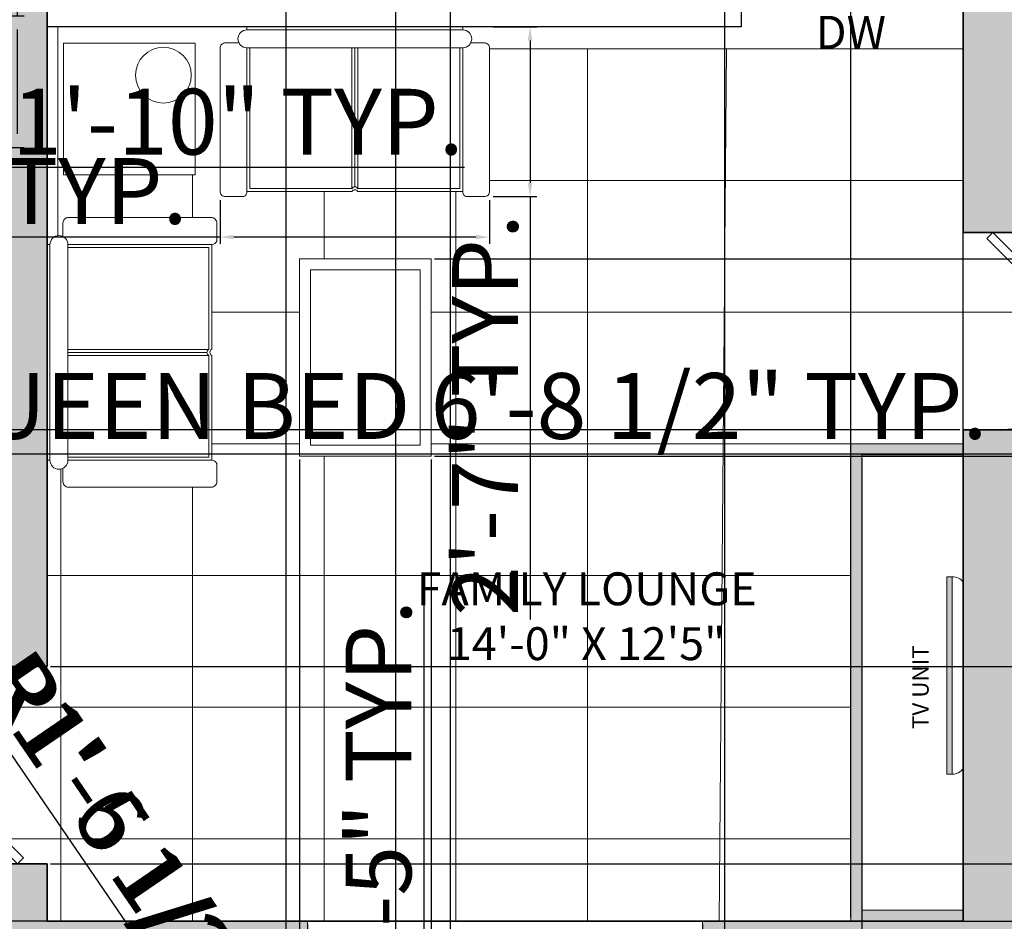
# Model space of a CAD drawing. Units: millimetres. Extents: x 542930 to 543750, y 628093 to 628738.
# Tile 6 of 14: x 543153 to 543333, y 628350 to 628514. Entities that reach past the tile are written whole.
import ezdxf

# ---------------------------------------------------------------- set-up
doc = ezdxf.new("R2010")
doc.units = ezdxf.units.MM
for name, color, linetype, lineweight in [('A-ANNO-DIMS', 2, 'Continuous', 18), ('A-EQPM', 9, 'Continuous', 18), ('A-EQPM-PATT', 9, 'Continuous', 13), ('A-FLOR-STRS', 7, 'Continuous', 25), ('A-FURN', 8, 'Continuous', 18), ('A-FURN-MILL', 8, 'Continuous', 18), ('A-FURN-PATT', 9, 'Continuous', 13), ('A-WALL', 7, 'Continuous', 35), ('DOORS', 30, 'Continuous', 18)]:
    doc.layers.add(name, color=color, linetype=linetype, lineweight=lineweight)
for name, color, linetype, lineweight, true_color in [('A-ANNO-TEXT', 40, 'Continuous', 18, 0xf8d731), ('A-AREA-IDEN', 40, 'Continuous', 18, 0xf8d731), ('A-FLOR-PATT', 241, 'Continuous', 13, 0xf7abae), ('A-WALL-PATT', 251, 'Continuous', 13, 0x636466)]:
    doc.layers.add(name, color=color, linetype=linetype, lineweight=lineweight, true_color=true_color)
doc.styles.get("Standard").update_dxf_attribs({"font": 'arial.ttf'})
doc.dimstyles.new('ISO-25', dxfattribs={"dimtxt": 12, "dimasz": 2.5, "dimexe": 1.25, "dimexo": 0.625, "dimtad": 1, "dimdec": 0, "dimlunit": 3, "dimtxsty": 'Standard', "dimcen": 2.5, "dimadec": 0, "dimazin": 0, "dimtfac": 1, "dimtdec": 0, "dimtmove": 0, "dimatfit": 3, "dimfxl": 1, "dimarcsym": 0})

# ---------------------------------------------------------------- blocks, each defined once
blk = doc.blocks.new('*U2')
for p, q in [((0, 0), (0, -6)), ((40, 0), (40, -6))]:
    blk.add_line(p, q)
blk.add_lwpolyline([(0, 0), (28.28, 28.28), (29.52, 27.05), (1.24, -1.24)], close=True)
blk.add_arc((0, 0), 40, 0, 45)
blk = doc.blocks.new('*U4')
for p, q in [((0, 0), (0, -6)), ((40, 0), (40, -6))]:
    blk.add_line(p, q)
blk.add_lwpolyline([(0, 0), (28.28, 28.28), (29.52, 27.05), (1.24, -1.24)], close=True)
blk.add_arc((0, 0), 40, 0, 45)
blk = doc.blocks.new('sofa')
for p, q in [((543001.62, 628230.38), (543001.62, 628182.38)), ((543010.62, 628230.38), (543045.62, 628230.38)), ((543091.62, 628230.38), (543091.62, 628182.38)), ((543045.62, 628229.38), (543045.62, 628182.38)), ((543046.62, 628228.78), (543046.62, 628182.38)), ((543010.62, 628176.38), (543082.62, 628176.38))]:
    blk.add_line(p, q)
for points in [[(543009.53, 628232.06), (543003.46, 628232.06, 0.414214), (543001.62, 628230.23)], [(543045.62, 628230.38, 0.623864), (543047.62, 628230.38), (543082.62, 628230.38), (543082.62, 628182.38), (543010.62, 628182.38), (543010.62, 628230.38, 0.297291), (543009.53, 628232.06)], [(543083.72, 628232.06, 0.297291), (543082.62, 628230.38), (543082.62, 628182.38)], [(543091.62, 628230.23, 0.414214), (543089.79, 628232.06), (543083.72, 628232.06)], [(543001.62, 628182.54, 0.414214), (543003.46, 628180.7), (543007.93, 628180.7)], [(543082.62, 628182.38, -1), (543082.62, 628176.38), (543082.62, 628175.38), (543010.62, 628175.38), (543010.62, 628176.38, -1), (543010.62, 628182.38)], [(543085.32, 628180.7), (543089.79, 628180.7, 0.414214), (543091.62, 628182.54)]]:
    blk.add_lwpolyline(points, format="xyb")
for points in [[(543011.62, 628182.38), (543011.62, 628229.38), (543045.62, 628229.38), (543045.62, 628229.4)], [(543047.62, 628182.38), (543047.62, 628229.38), (543047.62, 628229.4)], [(543047.62, 628229.38), (543081.62, 628229.38), (543081.62, 628182.38)]]:
    blk.add_lwpolyline(points)
blk.add_arc((543046.62, 628229.89), 1.11, 206.0829, 333.9171)
blk = doc.blocks.new('*D33')
at = {"layer": 'A-ANNO-DIMS', "color": 0, "lineweight": -2, "transparency": 16777216}
for p, q in [((543189.7, 628481.25), (543189.7, 628473.25)), ((543238.84, 628481.25), (543238.84, 628473.25)), ((543189.7, 628474.5), (543062.56, 628474.5)), ((543236.34, 628474.5), (543192.2, 628474.5))]:
    blk.add_line(p, q, dxfattribs=at)
at = {"layer": 'A-ANNO-DIMS', "color": 0, "transparency": 16777216}
for points in [[(543192.2, 628474.92), (543192.2, 628474.09), (543189.7, 628474.5)], [(543236.34, 628474.92), (543236.34, 628474.09), (543238.84, 628474.5)]]:
    blk.add_solid(points, dxfattribs=at)
at = {"layer": 'Defpoints', "color": 0, "transparency": 16777216}
for p in [(543189.7, 628481.87), (543238.84, 628481.87), (543189.7, 628474.5)]:
    blk.add_point(p, dxfattribs=at)
at = {"layer": 'A-ANNO-DIMS', "color": 0, "transparency": 16777216, "insert": (543124.88, 628481.34), "char_height": 12, "attachment_point": 5}
blk.add_mtext('SOFA 4\'-1" TYP.', dxfattribs=at)
blk = doc.blocks.new('*D34')
at = {"layer": 'A-ANNO-DIMS', "color": 0, "lineweight": -2, "transparency": 16777216}
for p, q in [((543239.47, 628512.83), (543247.47, 628512.83)), ((543246.22, 628510.33), (543246.22, 628484.37)), ((543239.47, 628481.87), (543247.47, 628481.87)), ((543246.22, 628481.87), (543246.22, 628404.77))]:
    blk.add_line(p, q, dxfattribs=at)
at = {"layer": 'A-ANNO-DIMS', "color": 0, "transparency": 16777216}
for points in [[(543245.8, 628510.33), (543246.63, 628510.33), (543246.22, 628512.83)], [(543245.8, 628484.37), (543246.63, 628484.37), (543246.22, 628481.87)]]:
    blk.add_solid(points, dxfattribs=at)
at = {"layer": 'Defpoints', "color": 0, "transparency": 16777216}
for p in [(543238.84, 628512.83), (543238.84, 628481.87), (543246.22, 628481.87)]:
    blk.add_point(p, dxfattribs=at)
at = {"layer": 'A-ANNO-DIMS', "color": 0, "transparency": 16777216, "insert": (543239.56, 628442.07), "char_height": 12, "attachment_point": 5, "rotation": 90}
blk.add_mtext('2\'-7" TYP.', dxfattribs=at)
blk = doc.blocks.new('*D37')
at = {"layer": 'A-ANNO-DIMS', "color": 0, "lineweight": -2, "transparency": 16777216}
for p, q in [((543337.17, 628423.55), (543337.17, 628436.21)), ((543417.44, 628423.55), (543417.44, 628436.21)), ((543337.17, 628434.96), (543128.93, 628434.96)), ((543414.94, 628434.96), (543339.67, 628434.96))]:
    blk.add_line(p, q, dxfattribs=at)
at = {"layer": 'A-ANNO-DIMS', "color": 0, "transparency": 16777216}
for points in [[(543339.67, 628435.38), (543339.67, 628434.55), (543337.17, 628434.96)], [(543414.94, 628435.38), (543414.94, 628434.55), (543417.44, 628434.96)]]:
    blk.add_solid(points, dxfattribs=at)
at = {"layer": 'Defpoints', "color": 0, "transparency": 16777216}
for p in [(543337.17, 628434.96), (543337.17, 628422.92), (543417.44, 628422.92)]:
    blk.add_point(p, dxfattribs=at)
at = {"layer": 'A-ANNO-DIMS', "color": 0, "transparency": 16777216, "insert": (543231.8, 628442.16), "char_height": 12, "attachment_point": 5}
blk.add_mtext('QUEEN BED 6\'-8 1/2" TYP.', dxfattribs=at)
blk = doc.blocks.new('*D42')
at = {"layer": 'A-ANNO-DIMS', "color": 0, "lineweight": -2, "transparency": 16777216}
for p, q in [((543226.89, 628332.06), (543226.89, 628408.95)), ((543221.13, 628332.06), (543228.14, 628332.06)), ((543226.89, 628293.55), (543226.89, 628329.56)), ((543221.13, 628291.05), (543228.14, 628291.05))]:
    blk.add_line(p, q, dxfattribs=at)
at = {"layer": 'A-ANNO-DIMS', "color": 0, "transparency": 16777216}
for points in [[(543226.47, 628329.56), (543227.3, 628329.56), (543226.89, 628332.06)], [(543226.47, 628293.55), (543227.3, 628293.55), (543226.89, 628291.05)]]:
    blk.add_solid(points, dxfattribs=at)
at = {"layer": 'Defpoints', "color": 0, "transparency": 16777216}
for p in [(543220.5, 628332.06), (543226.89, 628332.06), (543220.5, 628291.05)]:
    blk.add_point(p, dxfattribs=at)
at = {"layer": 'A-ANNO-DIMS', "color": 0, "transparency": 16777216, "insert": (543220.13, 628371.75), "char_height": 12, "attachment_point": 5, "rotation": 90}
blk.add_mtext('3\'-5" TYP.', dxfattribs=at)
blk = doc.blocks.new('*D55')
at = {"layer": 'A-ANNO-DIMS', "color": 0, "lineweight": -2, "transparency": 16777216}
for p, q in [((543152.77, 628514.83), (543152.77, 628679.13)), ((543149.79, 628514.83), (543154.02, 628514.83)), ((543152.77, 628493.33), (543152.77, 628512.33)), ((543149.79, 628490.83), (543154.02, 628490.83))]:
    blk.add_line(p, q, dxfattribs=at)
at = {"layer": 'A-ANNO-DIMS', "color": 0, "transparency": 16777216}
for points in [[(543152.35, 628512.33), (543153.18, 628512.33), (543152.77, 628514.83)], [(543152.35, 628493.33), (543153.18, 628493.33), (543152.77, 628490.83)]]:
    blk.add_solid(points, dxfattribs=at)
at = {"layer": 'Defpoints', "color": 0, "transparency": 16777216}
for p in [(543149.17, 628514.83), (543152.77, 628514.83), (543149.17, 628490.83)]:
    blk.add_point(p, dxfattribs=at)
at = {"layer": 'A-ANNO-DIMS', "color": 0, "transparency": 16777216, "insert": (543145.93, 628598.23), "char_height": 12, "attachment_point": 5, "rotation": 90}
blk.add_mtext('COUNTER 2\'-0" TYP.', dxfattribs=at)
blk = doc.blocks.new('*D56')
at = {"layer": 'A-ANNO-DIMS', "color": 0, "lineweight": -2, "transparency": 16777216}
for p, q in [((543127.17, 628490.2), (543127.17, 628485.98)), ((543149.17, 628490.2), (543149.17, 628485.98)), ((543129.67, 628487.23), (543146.67, 628487.23)), ((543149.17, 628487.23), (543234.26, 628487.23))]:
    blk.add_line(p, q, dxfattribs=at)
at = {"layer": 'A-ANNO-DIMS', "color": 0, "transparency": 16777216}
for points in [[(543129.67, 628487.64), (543129.67, 628486.81), (543127.17, 628487.23)], [(543146.67, 628487.64), (543146.67, 628486.81), (543149.17, 628487.23)]]:
    blk.add_solid(points, dxfattribs=at)
at = {"layer": 'Defpoints', "color": 0, "transparency": 16777216}
for p in [(543127.17, 628490.83), (543149.17, 628490.83), (543149.17, 628487.23)]:
    blk.add_point(p, dxfattribs=at)
at = {"layer": 'A-ANNO-DIMS', "color": 0, "transparency": 16777216, "insert": (543192.96, 628493.98), "char_height": 12, "attachment_point": 5}
blk.add_mtext('1\'-10" TYP.', dxfattribs=at)
blk = doc.blocks.new('*D71')
at = {"layer": 'A-ANNO-DIMS', "color": 0, "lineweight": -2, "transparency": 16777216}
for p, q in [((543201.67, 628544.2), (543201.67, 628103.84)), ((543281.67, 628544.2), (543281.67, 628103.84)), ((543204.17, 628105.09), (543279.17, 628105.09))]:
    blk.add_line(p, q, dxfattribs=at)
at = {"layer": 'A-ANNO-DIMS', "color": 0, "transparency": 16777216}
for points in [[(543204.17, 628105.5), (543204.17, 628104.67), (543201.67, 628105.09)], [(543279.17, 628105.5), (543279.17, 628104.67), (543281.67, 628105.09)]]:
    blk.add_solid(points, dxfattribs=at)
at = {"layer": 'Defpoints', "color": 0, "transparency": 16777216}
for p in [(543201.67, 628544.83), (543281.67, 628544.83), (543281.67, 628105.09)]:
    blk.add_point(p, dxfattribs=at)
at = {"layer": 'A-ANNO-DIMS', "color": 0, "transparency": 16777216, "insert": (543241.67, 628111.84), "char_height": 12, "attachment_point": 5}
blk.add_mtext('6\'-8"', dxfattribs=at)
blk = doc.blocks.new('*D73')
at = {"layer": 'A-ANNO-DIMS', "color": 0, "lineweight": -2, "transparency": 16777216}
for p, q in [((543158.79, 628396.23), (543537.81, 628396.23)), ((543536.56, 628362.73), (543536.56, 628393.73)), ((543158.79, 628360.23), (543537.81, 628360.23))]:
    blk.add_line(p, q, dxfattribs=at)
at = {"layer": 'A-ANNO-DIMS', "color": 0, "transparency": 16777216}
for points in [[(543536.15, 628393.73), (543536.98, 628393.73), (543536.56, 628396.23)], [(543536.15, 628362.73), (543536.98, 628362.73), (543536.56, 628360.23)]]:
    blk.add_solid(points, dxfattribs=at)
at = {"layer": 'Defpoints', "color": 0, "transparency": 16777216}
for p in [(543158.17, 628396.23), (543536.56, 628396.23), (543158.17, 628360.23)]:
    blk.add_point(p, dxfattribs=at)
at = {"layer": 'A-ANNO-DIMS', "color": 0, "transparency": 16777216, "insert": (543529.81, 628378.23), "char_height": 12, "attachment_point": 5, "rotation": 90}
blk.add_mtext('3\'-0"', dxfattribs=at)
blk = doc.blocks.new('*D74')
at = {"layer": 'A-ANNO-DIMS', "color": 0, "lineweight": -2, "transparency": 16777216}
for p, q in [((543536.56, 628360.23), (543536.56, 628433.16)), ((543158.79, 628360.23), (543537.81, 628360.23)), ((543536.56, 628352.33), (543536.56, 628357.73)), ((543158.79, 628349.83), (543537.81, 628349.83))]:
    blk.add_line(p, q, dxfattribs=at)
at = {"layer": 'A-ANNO-DIMS', "color": 0, "transparency": 16777216}
for points in [[(543536.15, 628357.73), (543536.98, 628357.73), (543536.56, 628360.23)], [(543536.15, 628352.33), (543536.98, 628352.33), (543536.56, 628349.83)]]:
    blk.add_solid(points, dxfattribs=at)
at = {"layer": 'Defpoints', "color": 0, "transparency": 16777216}
for p in [(543158.17, 628360.23), (543536.56, 628360.23), (543158.17, 628349.83)]:
    blk.add_point(p, dxfattribs=at)
at = {"layer": 'A-ANNO-DIMS', "color": 0, "transparency": 16777216, "insert": (543529.73, 628397.95), "char_height": 12, "attachment_point": 5, "rotation": 90}
blk.add_mtext('0\'-10 1/2"', dxfattribs=at)
blk = doc.blocks.new('*D75')
at = {"layer": 'A-ANNO-DIMS', "color": 0, "lineweight": -2, "transparency": 16777216}
for p, q in [((543324.54, 628439.36), (542953.72, 628439.36)), ((542954.97, 628352.33), (542954.97, 628436.86)), ((543324.54, 628349.83), (542953.72, 628349.83))]:
    blk.add_line(p, q, dxfattribs=at)
at = {"layer": 'A-ANNO-DIMS', "color": 0, "transparency": 16777216}
for points in [[(542954.55, 628436.86), (542955.38, 628436.86), (542954.97, 628439.36)], [(542954.55, 628352.33), (542955.38, 628352.33), (542954.97, 628349.83)]]:
    blk.add_solid(points, dxfattribs=at)
at = {"layer": 'Defpoints', "color": 0, "transparency": 16777216}
for p in [(542954.97, 628439.36), (543325.17, 628439.36), (543325.17, 628349.83)]:
    blk.add_point(p, dxfattribs=at)
at = {"layer": 'A-ANNO-DIMS', "color": 0, "transparency": 16777216, "insert": (542948.14, 628394.6), "char_height": 12, "attachment_point": 5, "rotation": 90}
blk.add_mtext('7\'-5 1/2"', dxfattribs=at)
blk = doc.blocks.new('*D76')
at = {"layer": 'A-ANNO-DIMS', "color": 0, "lineweight": -2, "transparency": 16777216}
for p, q in [((543205.67, 628349.2), (543205.67, 628103.84)), ((543277.67, 628349.2), (543277.67, 628103.84)), ((543208.17, 628105.09), (543275.17, 628105.09))]:
    blk.add_line(p, q, dxfattribs=at)
at = {"layer": 'A-ANNO-DIMS', "color": 0, "transparency": 16777216}
for points in [[(543208.17, 628105.5), (543208.17, 628104.67), (543205.67, 628105.09)], [(543275.17, 628105.5), (543275.17, 628104.67), (543277.67, 628105.09)]]:
    blk.add_solid(points, dxfattribs=at)
at = {"layer": 'Defpoints', "color": 0, "transparency": 16777216}
for p in [(543205.67, 628349.83), (543277.67, 628349.83), (543277.67, 628105.09)]:
    blk.add_point(p, dxfattribs=at)
at = {"layer": 'A-ANNO-DIMS', "color": 0, "transparency": 16777216, "insert": (543241.67, 628111.84), "char_height": 12, "attachment_point": 5}
blk.add_mtext('6\'-0"', dxfattribs=at)
blk = doc.blocks.new('*D78')
at = {"layer": 'A-ANNO-DIMS', "color": 0, "lineweight": -2, "transparency": 16777216}
for p, q in [((543304.67, 628350.45), (543304.67, 628619.78)), ((543307.17, 628618.53), (543322.67, 628618.53)), ((543325.17, 628350.45), (543325.17, 628619.78)), ((543325.17, 628618.53), (543387.65, 628618.53))]:
    blk.add_line(p, q, dxfattribs=at)
at = {"layer": 'A-ANNO-DIMS', "color": 0, "transparency": 16777216}
for points in [[(543307.17, 628618.94), (543307.17, 628618.11), (543304.67, 628618.53)], [(543322.67, 628618.94), (543322.67, 628618.11), (543325.17, 628618.53)]]:
    blk.add_solid(points, dxfattribs=at)
at = {"layer": 'Defpoints', "color": 0, "transparency": 16777216}
for p in [(543325.17, 628618.53), (543304.67, 628349.83), (543325.17, 628349.83)]:
    blk.add_point(p, dxfattribs=at)
at = {"layer": 'A-ANNO-DIMS', "color": 0, "transparency": 16777216, "insert": (543357.66, 628625.36), "char_height": 12, "attachment_point": 5}
blk.add_mtext('1\'-8 1/2"', dxfattribs=at)
blk = doc.blocks.new('*D79')
at = {"layer": 'A-ANNO-DIMS', "color": 0, "lineweight": -2, "transparency": 16777216}
for p, q in [((543204.19, 628433.96), (543204.19, 628103.84)), ((543228.16, 628433.96), (543228.16, 628103.84)), ((543206.69, 628105.09), (543225.66, 628105.09)), ((543228.16, 628105.09), (543264.02, 628105.09))]:
    blk.add_line(p, q, dxfattribs=at)
at = {"layer": 'A-ANNO-DIMS', "color": 0, "transparency": 16777216}
for points in [[(543206.69, 628105.5), (543206.69, 628104.67), (543204.19, 628105.09)], [(543225.66, 628105.5), (543225.66, 628104.67), (543228.16, 628105.09)]]:
    blk.add_solid(points, dxfattribs=at)
at = {"layer": 'Defpoints', "color": 0, "transparency": 16777216}
for p in [(543204.19, 628434.59), (543228.16, 628434.59), (543228.16, 628105.09)]:
    blk.add_point(p, dxfattribs=at)
at = {"layer": 'A-ANNO-DIMS', "color": 0, "transparency": 16777216, "insert": (543247.34, 628111.84), "char_height": 12, "attachment_point": 5}
blk.add_mtext('2\'-0"', dxfattribs=at)
blk = doc.blocks.new('*D80')
at = {"layer": 'A-ANNO-DIMS', "color": 0, "lineweight": -2, "transparency": 16777216}
for p, q in [((543228.79, 628470.52), (543537.81, 628470.52)), ((543536.56, 628437.09), (543536.56, 628468.02)), ((543228.79, 628434.59), (543537.81, 628434.59))]:
    blk.add_line(p, q, dxfattribs=at)
at = {"layer": 'A-ANNO-DIMS', "color": 0, "transparency": 16777216}
for points in [[(543536.15, 628468.02), (543536.98, 628468.02), (543536.56, 628470.52)], [(543536.15, 628437.09), (543536.98, 628437.09), (543536.56, 628434.59)]]:
    blk.add_solid(points, dxfattribs=at)
at = {"layer": 'Defpoints', "color": 0, "transparency": 16777216}
for p in [(543228.16, 628470.52), (543536.56, 628470.52), (543228.16, 628434.59)]:
    blk.add_point(p, dxfattribs=at)
at = {"layer": 'A-ANNO-DIMS', "color": 0, "transparency": 16777216, "insert": (543529.81, 628452.55), "char_height": 12, "attachment_point": 5, "rotation": 90}
blk.add_mtext('3\'-0"', dxfattribs=at)
blk = doc.blocks.new('*D81')
at = {"layer": 'A-ANNO-DIMS', "color": 0, "lineweight": -2, "transparency": 16777216}
for p, q in [((543228.16, 628433.96), (543228.16, 628103.84)), ((543306.67, 628434.2), (543306.67, 628103.84)), ((543230.66, 628105.09), (543304.17, 628105.09))]:
    blk.add_line(p, q, dxfattribs=at)
at = {"layer": 'A-ANNO-DIMS', "color": 0, "transparency": 16777216}
for points in [[(543230.66, 628105.5), (543230.66, 628104.67), (543228.16, 628105.09)], [(543304.17, 628105.5), (543304.17, 628104.67), (543306.67, 628105.09)]]:
    blk.add_solid(points, dxfattribs=at)
at = {"layer": 'Defpoints', "color": 0, "transparency": 16777216}
for p in [(543228.16, 628434.59), (543306.67, 628434.83), (543306.67, 628105.09)]:
    blk.add_point(p, dxfattribs=at)
at = {"layer": 'A-ANNO-DIMS', "color": 0, "transparency": 16777216, "insert": (543267.41, 628111.92), "char_height": 12, "attachment_point": 5}
blk.add_mtext('6\'-6 1/2"', dxfattribs=at)
blk = doc.blocks.new('*D87')
at = {"layer": 'A-ANNO-DIMS', "color": 0, "lineweight": -2, "transparency": 16777216}
for p, q in [((543221.67, 628580.2), (543221.67, 628103.84)), ((543231.67, 628580.2), (543231.67, 628103.84)), ((543224.17, 628105.09), (543229.17, 628105.09)), ((543231.67, 628105.09), (543276.64, 628105.09))]:
    blk.add_line(p, q, dxfattribs=at)
at = {"layer": 'A-ANNO-DIMS', "color": 0, "transparency": 16777216}
for points in [[(543224.17, 628105.5), (543224.17, 628104.67), (543221.67, 628105.09)], [(543229.17, 628105.5), (543229.17, 628104.67), (543231.67, 628105.09)]]:
    blk.add_solid(points, dxfattribs=at)
at = {"layer": 'Defpoints', "color": 0, "transparency": 16777216}
for p in [(543221.67, 628580.83), (543231.67, 628580.83), (543231.67, 628105.09)]:
    blk.add_point(p, dxfattribs=at)
at = {"layer": 'A-ANNO-DIMS', "color": 0, "transparency": 16777216, "insert": (543255.4, 628111.84), "char_height": 12, "attachment_point": 5}
blk.add_mtext('0\'-10"', dxfattribs=at)
blk = doc.blocks.new('*D92')
at = {"layer": 'A-ANNO-DIMS', "color": 0, "lineweight": -2, "transparency": 16777216}
for p, q in [((543166.68, 628358.16), (543206.81, 628299.51)), ((543246.12, 628242.05), (543208.22, 628297.45))]:
    blk.add_line(p, q, dxfattribs=at)
at = {"layer": 'A-ANNO-DIMS', "color": 0, "transparency": 16777216}
blk.add_solid([(543208.57, 628297.68), (543207.88, 628297.21), (543206.81, 628299.51)], dxfattribs=at)
at = {"layer": 'Defpoints', "color": 0, "transparency": 16777216}
for p in [(543166.68, 628358.16), (543206.81, 628299.51)]:
    blk.add_point(p, dxfattribs=at)
at = {"layer": 'A-ANNO-DIMS', "color": 0, "transparency": 16777216, "insert": (543236.46, 628268.13), "char_height": 12, "attachment_point": 5, "rotation": 304.379}
blk.add_mtext('R5\'-11"', dxfattribs=at)
blk = doc.blocks.new('*D94')
at = {"layer": 'A-ANNO-DIMS', "color": 0, "lineweight": -2, "transparency": 16777216}
for p, q in [((543143.96, 628391.37), (543186.37, 628329.39)), ((543198.34, 628311.9), (543187.78, 628327.33))]:
    blk.add_line(p, q, dxfattribs=at)
at = {"layer": 'A-ANNO-DIMS', "color": 0, "transparency": 16777216}
blk.add_solid([(543186.71, 628329.63), (543186.02, 628329.15), (543187.78, 628327.33)], dxfattribs=at)
at = {"layer": 'Defpoints', "color": 0, "transparency": 16777216}
for p in [(543187.78, 628327.33), (543198.34, 628311.9)]:
    blk.add_point(p, dxfattribs=at)
at = {"layer": 'A-ANNO-DIMS', "color": 0, "transparency": 16777216, "insert": (543170.1, 628365.27), "char_height": 12, "attachment_point": 5, "rotation": 304.3793}
blk.add_mtext('R1\'-6 1/2"', dxfattribs=at)
blk = doc.blocks.new('*D95')
at = {"layer": 'A-ANNO-DIMS', "color": 0, "lineweight": -2, "transparency": 16777216}
for p, q in [((543144.53, 628390.54), (543186.93, 628328.57)), ((543198.34, 628311.9), (543188.34, 628326.5))]:
    blk.add_line(p, q, dxfattribs=at)
at = {"layer": 'A-ANNO-DIMS', "color": 0, "transparency": 16777216}
blk.add_solid([(543187.28, 628328.8), (543186.59, 628328.33), (543188.34, 628326.5)], dxfattribs=at)
at = {"layer": 'Defpoints', "color": 0, "transparency": 16777216}
for p in [(543188.34, 628326.5), (543198.34, 628311.9)]:
    blk.add_point(p, dxfattribs=at)
at = {"layer": 'A-ANNO-DIMS', "color": 0, "transparency": 16777216, "insert": (543170.66, 628364.44), "char_height": 12, "attachment_point": 5, "rotation": 304.3778}
blk.add_mtext('R1\'-5 1/2"', dxfattribs=at)

msp = doc.modelspace()

# ---------------------------------------------------------------- hatches: boundary and pattern name
at = {"layer": 'A-EQPM-PATT'}
h = msp.add_hatch(color=256, dxfattribs=at)
h.dxf.hatch_style = 1
h.paths.add_polyline_path([(543323.17, 628412.6), (543322.17, 628412.6), (543322.17, 628376.6), (543323.17, 628376.6)])
at = {"layer": 'A-FURN-PATT'}
h = msp.add_hatch(color=256, dxfattribs=at)
h.dxf.hatch_style = 1
h.paths.add_polyline_path([(543306.67, 628434.83), (543325.17, 628434.83), (543325.17, 628436.83), (543304.67, 628436.83), (543304.67, 628349.83), (543325.17, 628349.83), (543325.17, 628351.83), (543306.67, 628351.83)])
at = {"layer": 'A-WALL-PATT'}
h = msp.add_hatch(color=256, dxfattribs=at)
h.dxf.hatch_style = 1
h.paths.add_polyline_path([(543158.17, 628580.83), (543211.67, 628580.83), (543211.67, 628589.83), (543137.07, 628589.83), (543137.07, 628580.83), (543149.17, 628580.83), (543149.17, 628490.83), (543073.17, 628490.83), (543073.17, 628496.14), (543068.67, 628496.14), (543068.67, 628490.83), (543064.67, 628490.83), (543064.67, 628481.83), (543149.17, 628481.83), (543149.17, 628396.23), (543158.17, 628396.23)])
h = msp.add_hatch(color=256, dxfattribs=at)
h.dxf.hatch_style = 1
h.paths.add_polyline_path([(543454.53, 628589.83), (543271.67, 628589.83), (543271.67, 628580.83), (543325.17, 628580.83), (543325.17, 628475.36), (543334.17, 628475.36), (543334.17, 628481.83), (543370.17, 628481.83), (543370.17, 628490.83), (543334.17, 628490.83), (543334.17, 628580.83), (543410.17, 628580.83), (543410.17, 628524.86), (543414.67, 628524.86), (543414.67, 628580.83), (543454.53, 628580.83)])
h = msp.add_hatch(color=256, dxfattribs=at)
h.dxf.hatch_style = 1
h.paths.add_polyline_path([(543388.65, 628262.83), (543374.28, 628262.83), (543334.17, 628262.83), (543334.17, 628439.36), (543325.17, 628439.36), (543325.17, 628349.83), (543277.67, 628349.83), (543277.67, 628340.83), (543325.17, 628340.83), (543325.17, 628253.83), (543388.65, 628253.83)])
h = msp.add_hatch(color=256, dxfattribs=at)
h.dxf.hatch_style = 1
h.paths.add_polyline_path([(543158.17, 628340.83), (543205.67, 628340.83), (543205.67, 628349.83), (543158.17, 628349.83), (543158.17, 628360.23), (543149.17, 628360.23), (543149.17, 628262.83), (543094.69, 628262.83), (543094.69, 628253.83), (543158.17, 628253.83)])

# ---------------------------------------------------------------- linework, layer by layer
at = {"layer": 'A-EQPM'}
for p, q in [((543322.17, 628376.6), (543322.17, 628412.6)), ((543322.17, 628412.6), (543323.17, 628412.6)), ((543323.17, 628376.6), (543323.17, 628412.6)), ((543322.17, 628376.6), (543323.17, 628376.6))]:
    msp.add_line(p, q, dxfattribs=at)
for centre, start, end in [((543323.1, 628409.96), 38.3608, 88.5091), ((543323.1, 628379.23), 271.4909, 321.6392)]:
    msp.add_arc(centre, 2.64, start, end, dxfattribs=at)
at = {"layer": 'A-FLOR-PATT'}
for p, q in [((543160.17, 628474.75), (543160.17, 628512.83)), ((543238.84, 628508.83), (543325.17, 628508.83)), ((543256.67, 628349.83), (543256.67, 628508.83)), ((543280.67, 628349.83), (543282.01, 628508.83)), ((543304.67, 628436.83), (543304.67, 628508.83)), ((543184.67, 628478.05), (543184.67, 628485.83)), ((543238.84, 628484.83), (543325.17, 628484.83)), ((543208.67, 628470.52), (543208.67, 628482.79)), ((543232.67, 628349.83), (543232.67, 628482.79)), ((543188.2, 628460.83), (543204.19, 628460.83)), ((543228.16, 628460.83), (543406.17, 628460.83)), ((543188.2, 628436.83), (543204.19, 628436.83)), ((543228.16, 628436.83), (543304.67, 628436.83)), ((543208.67, 628349.83), (543208.67, 628434.59)), ((543160.67, 628349.83), (543160.67, 628432.22)), ((543184.67, 628349.83), (543184.67, 628428.91)), ((543158.17, 628412.83), (543304.67, 628412.83)), ((543077.27, 628388.83), (543304.67, 628388.83)), ((543077.27, 628364.83), (543304.67, 628364.83))]:
    msp.add_line(p, q, dxfattribs=at)
at = {"layer": 'A-FLOR-STRS'}
for p, q in [((543284.67, 628547.83), (543284.67, 628512.83)), ((543284.67, 628512.83), (543158.17, 628512.83))]:
    msp.add_line(p, q, dxfattribs=at)
at = {"layer": 'A-FURN'}
for p, q in [((543185.17, 628509.83), (543161.17, 628509.83)), ((543161.17, 628485.83), (543161.17, 628509.83)), ((543185.17, 628485.83), (543185.17, 628509.83)), ((543185.17, 628485.83), (543161.17, 628485.83))]:
    msp.add_line(p, q, dxfattribs=at)
for points in [[(543204.19, 628470.52), (543228.16, 628470.52), (543228.16, 628434.59), (543204.19, 628434.59)], [(543206.19, 628468.52), (543226.16, 628468.52), (543226.16, 628436.59), (543206.19, 628436.59)]]:
    msp.add_lwpolyline(points, close=True, dxfattribs=at)
msp.add_circle((543179.38, 628504.02), 5.08, dxfattribs=at)
at = {"layer": 'A-FURN-MILL'}
for p, q in [((543304.67, 628349.83), (543304.67, 628436.83)), ((543304.67, 628436.83), (543325.17, 628436.83)), ((543306.67, 628351.83), (543306.67, 628434.83)), ((543306.67, 628434.83), (543325.17, 628434.83)), ((543325.17, 628351.83), (543306.67, 628351.83))]:
    msp.add_line(p, q, dxfattribs=at)
at = {"layer": 'A-WALL'}
for p, q in [((543158.17, 628396.23), (543158.17, 628580.83)), ((543325.17, 628475.36), (543325.17, 628580.83)), ((543334.17, 628475.36), (543325.17, 628475.36)), ((543325.17, 628349.83), (543325.17, 628439.36)), ((543334.17, 628439.36), (543325.17, 628439.36)), ((543158.17, 628396.23), (543149.17, 628396.23)), ((543158.17, 628360.23), (543149.17, 628360.23)), ((543158.17, 628349.83), (543158.17, 628360.23)), ((543325.17, 628349.83), (543158.17, 628349.83))]:
    msp.add_line(p, q, dxfattribs=at)
at = {"layer": 'DOORS'}
for p, q in [((543205.67, 628349.83), (543205.67, 628340.83)), ((543277.67, 628349.83), (543277.67, 628340.83))]:
    msp.add_line(p, q, dxfattribs=at)

# ---------------------------------------------------------------- block references
at = {"layer": 'A-FURN', "xscale": 0.5460747824189197, "yscale": 0.5460747824189197, "zscale": 0.5460747824189197}
for p, rotation in [((839758.34, 971543.56), 180), ((200127.43, 924997.55), 270)]:
    msp.add_blockref('sofa', p, dxfattribs=dict(at, rotation=rotation))
at = {"layer": 'DOORS'}
for name, p, xscale, yscale, zscale, rotation in [('*U2', (543330.57, 628475.36), 0.8999999999970896, 0.8999999999970896, 0.8999999999970896, 270), ('*U4', (543152.77, 628360.23), 0.9000000000029102, 0.9000000000029102, 0.9000000000029102, 90)]:
    msp.add_blockref(name, p, dxfattribs=dict(at, xscale=xscale, yscale=yscale, zscale=zscale, rotation=rotation))

# ---------------------------------------------------------------- texts
at = {"layer": 'A-ANNO-TEXT', "insert": (543294.61, 628514.83), "char_height": 6, "attachment_point": 1}
msp.add_mtext_dynamic_manual_height_columns('  DW', width=44.748, gutter_width=12.5, heights=[0], dxfattribs=at)
at = {"layer": 'A-ANNO-TEXT', "insert": (543315.87, 628382.98), "char_height": 3, "attachment_point": 1, "rotation": 90}
msp.add_mtext_dynamic_manual_height_columns('  TV UNIT', width=44.748, gutter_width=12.5, heights=[0], dxfattribs=at)
at = {"layer": 'A-AREA-IDEN', "insert": (543221.88, 628413.39), "char_height": 6, "attachment_point": 1}
msp.add_mtext_dynamic_manual_height_columns('  FAMILY LOUNGE\\P     14\'-0" X 12\'5"', width=77.2525, gutter_width=12.5, heights=[0], dxfattribs=at)

# ---------------------------------------------------------------- dimensions: what is measured, and where the dimension line sits
at = {"layer": 'A-ANNO-DIMS'}
for base, p1, p2, angle, text, picture, middle in [((543152.77, 628514.83), (543149.17, 628490.83), (543149.17, 628514.83), 90, 'COUNTER <> TYP.', '*D55', (543145.93, 628598.23)), ((543246.22, 628481.87), (543238.84, 628512.83), (543238.84, 628481.87), 270, '<> TYP.', '*D34', (543239.56, 628442.07)), ((543189.7, 628474.5), (543238.84, 628481.87), (543189.7, 628481.87), 180, 'SOFA <> TYP.', '*D33', (543124.88, 628481.34)), ((543337.17, 628434.96), (543417.44, 628422.92), (543337.17, 628422.92), 180, 'QUEEN BED <> TYP.', '*D37', (543231.8, 628442.16)), ((543226.89, 628332.06), (543220.5, 628291.05), (543220.5, 628332.06), 90, '<> TYP.', '*D42', (543220.13, 628371.75))]:
    dim = msp.add_linear_dim(base=base, p1=p1, p2=p2, angle=angle, text=text, dimstyle='ISO-25', override={"dimdec": 1, "dimlfac": 1, "dimrnd": 0, "dimzin": 1, "dimdsep": 46, "dimlunit": 4, "dimfrac": 2}, dxfattribs=at)
    dim.commit()
    dim.dimension.update_dxf_attribs({"geometry": picture, "text_midpoint": middle})
for base, p1, p2, picture, middle in [((543325.17, 628618.53), (543304.67, 628349.83), (543325.17, 628349.83), '*D78', (543357.66, 628625.36)), ((543231.67, 628105.09), (543221.67, 628580.83), (543231.67, 628580.83), '*D87', (543255.4, 628111.84)), ((543281.67, 628105.09), (543201.67, 628544.83), (543281.67, 628544.83), '*D71', (543241.67, 628111.84)), ((543228.16, 628105.09), (543204.19, 628434.59), (543228.16, 628434.59), '*D79', (543247.34, 628111.84)), ((543306.67, 628105.09), (543228.16, 628434.59), (543306.67, 628434.83), '*D81', (543267.41, 628111.92)), ((543277.67, 628105.09), (543205.67, 628349.83), (543277.67, 628349.83), '*D76', (543241.67, 628111.84))]:
    dim = msp.add_linear_dim(base=base, p1=p1, p2=p2, dimstyle='ISO-25', override={"dimdec": 1, "dimlfac": 1, "dimrnd": 0, "dimzin": 1, "dimdsep": 46, "dimlunit": 4, "dimfrac": 2}, dxfattribs=at)
    dim.commit()
    dim.dimension.update_dxf_attribs({"geometry": picture, "text_midpoint": middle})
dim = msp.add_linear_dim(base=(543149.17, 628487.23), p1=(543127.17, 628490.83), p2=(543149.17, 628490.83), text='<> TYP.', dimstyle='ISO-25', override={"dimdec": 1, "dimlfac": 1, "dimrnd": 0, "dimzin": 1, "dimdsep": 46, "dimlunit": 4, "dimfrac": 2}, dxfattribs=at)
dim.commit()
dim.dimension.update_dxf_attribs({"geometry": '*D56', "text_midpoint": (543192.96, 628493.98)})
for base, p1, p2, picture, middle in [((543536.56, 628470.52), (543228.16, 628434.59), (543228.16, 628470.52), '*D80', (543529.81, 628452.55)), ((542954.97, 628439.36), (543325.17, 628349.83), (543325.17, 628439.36), '*D75', (542948.14, 628394.6)), ((543536.56, 628360.23), (543158.17, 628349.83), (543158.17, 628360.23), '*D74', (543529.73, 628397.95)), ((543536.56, 628396.23), (543158.17, 628360.23), (543158.17, 628396.23), '*D73', (543529.81, 628378.23))]:
    dim = msp.add_linear_dim(base=base, p1=p1, p2=p2, angle=90, dimstyle='ISO-25', override={"dimdec": 1, "dimlfac": 1, "dimrnd": 0, "dimzin": 1, "dimdsep": 46, "dimlunit": 4, "dimfrac": 2}, dxfattribs=at)
    dim.commit()
    dim.dimension.update_dxf_attribs({"geometry": picture, "text_midpoint": middle})
for mpoint, picture, middle in [((543187.78, 628327.33), '*D94', (543170.1, 628365.27)), ((543188.34, 628326.5), '*D95', (543170.66, 628364.44))]:
    dim = msp.add_radius_dim(center=(543198.34, 628311.9), mpoint=mpoint, dimstyle='ISO-25', override={"dimdec": 1, "dimlfac": 1, "dimrnd": 0, "dimzin": 1, "dimdsep": 46, "dimlunit": 4, "dimfrac": 2}, dxfattribs=at)
    dim.commit()
    dim.dimension.update_dxf_attribs({"geometry": picture, "text_midpoint": middle})
dim = msp.add_radius_dim(center=(543166.68, 628358.16), mpoint=(543206.81, 628299.51), dimstyle='ISO-25', override={"dimdec": 1, "dimlfac": 1, "dimrnd": 0, "dimzin": 1, "dimdsep": 46, "dimlunit": 4, "dimfrac": 2}, dxfattribs=at)
dim.commit()
dim.dimension.update_dxf_attribs({"geometry": '*D92', "text_midpoint": (543230.89, 628264.32), "dimtype": 164})

doc.saveas('drawing.dxf')
